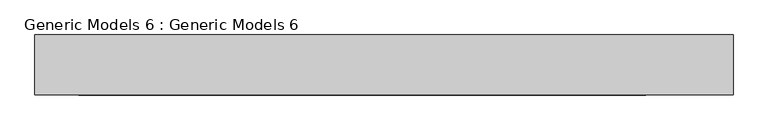
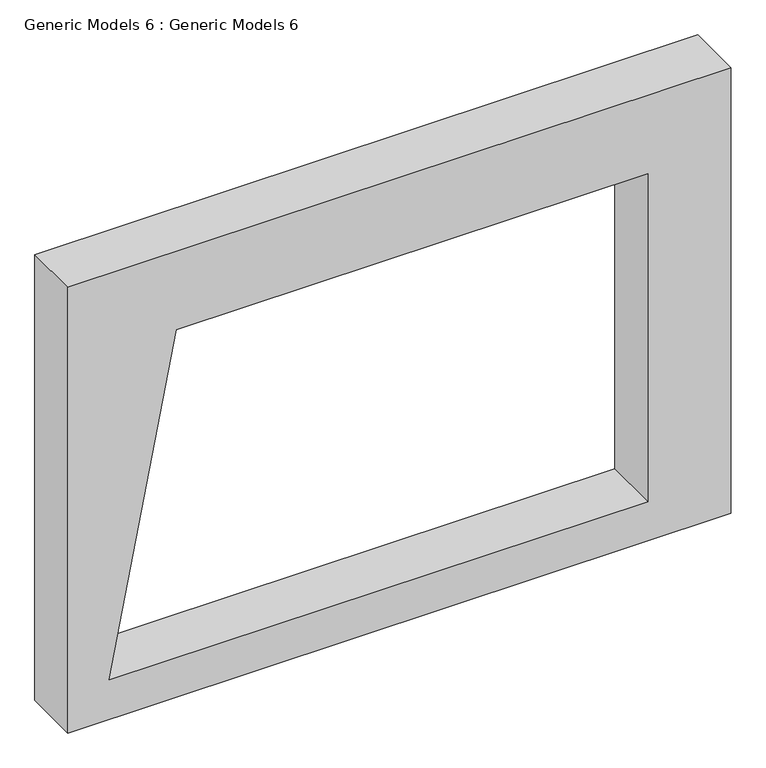
"""IFC4 building model written with IfcOpenShell, lengths in millimetres: proxy geometry, Generic Models 6 : Generic Models 6."""

from ifc_helpers import new_model, si_unit, frame, origin, place, context, project, spatial, polyline, outline, extrude, source, transform, mapped, element, save


def generic_models_6_generic_models_6_33fdfef5(model_context):
    return source(origin(), model_context, "Body", "SweptSolid", [
        extrude(outline(polyline([(6502.4, -4797.9586008), (3048.0, -4797.9586008), (3048.0, 66.1413992), (6502.4, 66.1413992), (6502.4, -4797.9586008)]), holes=[polyline([(5892.8, -3999.4326155), (5892.8, -543.4586008), (3352.8, -543.4586008), (3352.8, -4493.1586008), (5892.8, -3999.4326155)])]), frame((0.0, -7640.6478449, 0.0), z_axis=(0.0, 1.0, 0.0), x_axis=(0.0, 0.0, 1.0)), (0.0, 0.0, 1.0), 418.5355725),
    ])


if __name__ == "__main__":
    model = new_model("IFC4")
    model_context = context("Model", 3, world=origin())
    ifc_project = project(units=[si_unit("LENGTHUNIT", "METRE", prefix="MILLI")], contexts=[model_context])
    site = spatial("IfcSite", under=ifc_project)
    building = spatial("IfcBuilding", under=site)
    placement = place(None, origin())
    generic_models_6_generic_models_6_shape = generic_models_6_generic_models_6_33fdfef5(model_context)
    element("IfcBuildingElementProxy", 1, Name="Generic Models 6 : Generic Models 6", ObjectType="Generic Models 6 : Generic Models 6", at=placement, inside=building, context=model_context, shape_type="MappedRepresentation", body=[
        mapped(generic_models_6_generic_models_6_shape, transform((0.0, 0.0, 0.0), x_axis=(1.0, 0.0, 0.0), y_axis=(0.0, 1.0, 0.0), z_axis=(0.0, 0.0, 1.0))),
    ])
    save(model, "model.ifc")

# Revit data of these elements
# Element 1 (IfcBuildingElementProxy, "Generic Models 6 : Generic Models 6")
#   Materials on its faces: "feature frame"
# Materials
#   "feature frame": class "Generic", colour RGB 120 120 120, transparency 0, Cost = 0
